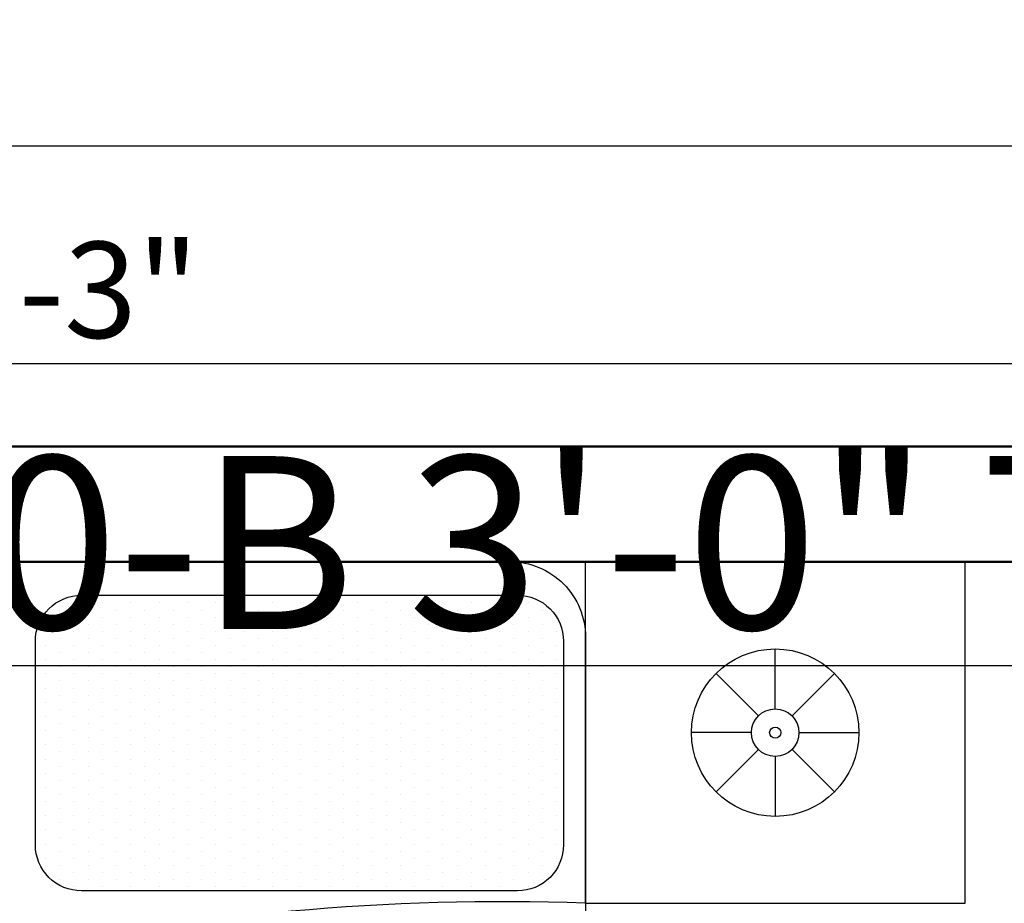
# Model space of a CAD drawing. Units: inches. Extents: x 3064 to 19385, y 846 to 15425.
# Tile 47 of 108: x 5430 to 5481, y 1368 to 1414. Entities that reach past the tile are written whole.
import ezdxf

# ---------------------------------------------------------------- set-up
doc = ezdxf.new("R2010")
doc.units = ezdxf.units.IN
for name, color, linetype, lineweight in [('A-ANNO-DIMS', 2, 'Continuous', 18), ('A-FLOR-FIXT', 9, 'Continuous', 18), ('A-WALL', 7, 'Continuous', 50)]:
    doc.layers.add(name, color=color, linetype=linetype, lineweight=lineweight)
doc.layers.add('BLOCK', color=6, linetype='Continuous')
doc.styles.get("Standard").update_dxf_attribs({"font": 'arial.ttf'})
doc.dimstyles.new('ISO-25', dxfattribs={"dimtxt": 9, "dimasz": 2.5, "dimexe": 1.25, "dimexo": 0.625, "dimtad": 1, "dimdec": 1, "dimlunit": 3, "dimtxsty": 'Standard', "dimcen": 2.5, "dimadec": 0, "dimazin": 0, "dimtfac": 1, "dimtdec": 1, "dimtmove": 0, "dimatfit": 3, "dimfxl": 1, "dimarcsym": 0})

# ---------------------------------------------------------------- blocks, each defined once
blk = doc.blocks.new('*X7')
at = {"color": 0}
for p, q in [((273.9375, 457.03125), (273.9375, 457.03125)), ((274.3125, 457.03125), (274.3125, 457.03125)), ((274.6875, 457.03125), (274.6875, 457.03125)), ((275.0625, 457.03125), (275.0625, 457.03125)), ((275.4375, 457.03125), (275.4375, 457.03125)), ((275.8125, 457.03125), (275.8125, 457.03125)), ((276.1875, 457.03125), (276.1875, 457.03125)), ((276.5625, 457.03125), (276.5625, 457.03125)), ((276.9375, 457.03125), (276.9375, 457.03125)), ((277.3125, 457.03125), (277.3125, 457.03125)), ((277.6875, 457.03125), (277.6875, 457.03125)), ((278.0625, 457.03125), (278.0625, 457.03125)), ((278.4375, 457.03125), (278.4375, 457.03125)), ((278.8125, 457.03125), (278.8125, 457.03125)), ((279.1875, 457.03125), (279.1875, 457.03125)), ((279.5625, 457.03125), (279.5625, 457.03125)), ((273.5625, 456.84375), (273.5625, 456.84375)), ((273.75, 456.9375), (273.75, 456.9375)), ((273.9375, 456.84375), (273.9375, 456.84375)), ((274.125, 456.9375), (274.125, 456.9375)), ((274.3125, 456.84375), (274.3125, 456.84375)), ((274.5, 456.9375), (274.5, 456.9375)), ((274.6875, 456.84375), (274.6875, 456.84375)), ((274.875, 456.9375), (274.875, 456.9375)), ((275.0625, 456.84375), (275.0625, 456.84375)), ((275.25, 456.9375), (275.25, 456.9375)), ((275.4375, 456.84375), (275.4375, 456.84375)), ((275.625, 456.9375), (275.625, 456.9375)), ((275.8125, 456.84375), (275.8125, 456.84375)), ((276, 456.9375), (276, 456.9375)), ((276.1875, 456.84375), (276.1875, 456.84375)), ((276.375, 456.9375), (276.375, 456.9375)), ((276.5625, 456.84375), (276.5625, 456.84375)), ((276.75, 456.9375), (276.75, 456.9375)), ((276.9375, 456.84375), (276.9375, 456.84375)), ((277.125, 456.9375), (277.125, 456.9375)), ((277.3125, 456.84375), (277.3125, 456.84375)), ((277.5, 456.9375), (277.5, 456.9375)), ((277.6875, 456.84375), (277.6875, 456.84375)), ((277.875, 456.9375), (277.875, 456.9375)), ((278.0625, 456.84375), (278.0625, 456.84375)), ((278.25, 456.9375), (278.25, 456.9375)), ((278.4375, 456.84375), (278.4375, 456.84375)), ((278.625, 456.9375), (278.625, 456.9375)), ((278.8125, 456.84375), (278.8125, 456.84375)), ((279, 456.9375), (279, 456.9375)), ((279.1875, 456.84375), (279.1875, 456.84375)), ((279.375, 456.9375), (279.375, 456.9375)), ((279.5625, 456.84375), (279.5625, 456.84375)), ((279.75, 456.9375), (279.75, 456.9375)), ((279.9375, 456.84375), (279.9375, 456.84375)), ((273.375, 456.75), (273.375, 456.75)), ((273.75, 456.75), (273.75, 456.75)), ((274.125, 456.75), (274.125, 456.75)), ((274.5, 456.75), (274.5, 456.75)), ((274.875, 456.75), (274.875, 456.75)), ((275.25, 456.75), (275.25, 456.75)), ((275.625, 456.75), (275.625, 456.75)), ((276, 456.75), (276, 456.75)), ((276.375, 456.75), (276.375, 456.75)), ((276.75, 456.75), (276.75, 456.75)), ((277.125, 456.75), (277.125, 456.75)), ((277.5, 456.75), (277.5, 456.75)), ((277.875, 456.75), (277.875, 456.75)), ((278.25, 456.75), (278.25, 456.75)), ((278.625, 456.75), (278.625, 456.75)), ((279, 456.75), (279, 456.75)), ((279.375, 456.75), (279.375, 456.75)), ((279.75, 456.75), (279.75, 456.75)), ((280.125, 456.75), (280.125, 456.75)), ((273.375, 456.5625), (273.375, 456.5625)), ((273.5625, 456.65625), (273.5625, 456.65625)), ((273.75, 456.5625), (273.75, 456.5625)), ((273.9375, 456.65625), (273.9375, 456.65625)), ((274.125, 456.5625), (274.125, 456.5625)), ((274.3125, 456.65625), (274.3125, 456.65625)), ((274.5, 456.5625), (274.5, 456.5625)), ((274.6875, 456.65625), (274.6875, 456.65625)), ((274.875, 456.5625), (274.875, 456.5625)), ((275.0625, 456.65625), (275.0625, 456.65625)), ((275.25, 456.5625), (275.25, 456.5625)), ((275.4375, 456.65625), (275.4375, 456.65625)), ((275.625, 456.5625), (275.625, 456.5625)), ((275.8125, 456.65625), (275.8125, 456.65625)), ((276, 456.5625), (276, 456.5625)), ((276.1875, 456.65625), (276.1875, 456.65625)), ((276.375, 456.5625), (276.375, 456.5625)), ((276.5625, 456.65625), (276.5625, 456.65625)), ((276.75, 456.5625), (276.75, 456.5625)), ((276.9375, 456.65625), (276.9375, 456.65625)), ((277.125, 456.5625), (277.125, 456.5625)), ((277.3125, 456.65625), (277.3125, 456.65625)), ((277.5, 456.5625), (277.5, 456.5625)), ((277.6875, 456.65625), (277.6875, 456.65625)), ((277.875, 456.5625), (277.875, 456.5625)), ((278.0625, 456.65625), (278.0625, 456.65625)), ((278.25, 456.5625), (278.25, 456.5625)), ((278.4375, 456.65625), (278.4375, 456.65625)), ((278.625, 456.5625), (278.625, 456.5625)), ((278.8125, 456.65625), (278.8125, 456.65625)), ((279, 456.5625), (279, 456.5625)), ((279.1875, 456.65625), (279.1875, 456.65625)), ((279.375, 456.5625), (279.375, 456.5625)), ((279.5625, 456.65625), (279.5625, 456.65625)), ((279.75, 456.5625), (279.75, 456.5625)), ((279.9375, 456.65625), (279.9375, 456.65625)), ((280.125, 456.5625), (280.125, 456.5625)), ((273.5625, 456.46875), (273.5625, 456.46875)), ((273.9375, 456.46875), (273.9375, 456.46875)), ((274.3125, 456.46875), (274.3125, 456.46875)), ((274.6875, 456.46875), (274.6875, 456.46875)), ((275.0625, 456.46875), (275.0625, 456.46875)), ((275.4375, 456.46875), (275.4375, 456.46875)), ((275.8125, 456.46875), (275.8125, 456.46875)), ((276.1875, 456.46875), (276.1875, 456.46875)), ((276.5625, 456.46875), (276.5625, 456.46875)), ((276.9375, 456.46875), (276.9375, 456.46875)), ((277.3125, 456.46875), (277.3125, 456.46875)), ((277.6875, 456.46875), (277.6875, 456.46875)), ((278.0625, 456.46875), (278.0625, 456.46875)), ((278.4375, 456.46875), (278.4375, 456.46875)), ((278.8125, 456.46875), (278.8125, 456.46875)), ((279.1875, 456.46875), (279.1875, 456.46875)), ((279.5625, 456.46875), (279.5625, 456.46875)), ((279.9375, 456.46875), (279.9375, 456.46875)), ((273.375, 456.375), (273.375, 456.375)), ((273.75, 456.375), (273.75, 456.375)), ((274.125, 456.375), (274.125, 456.375)), ((274.5, 456.375), (274.5, 456.375)), ((274.875, 456.375), (274.875, 456.375)), ((275.25, 456.375), (275.25, 456.375)), ((275.625, 456.375), (275.625, 456.375)), ((276, 456.375), (276, 456.375)), ((276.375, 456.375), (276.375, 456.375)), ((276.75, 456.375), (276.75, 456.375)), ((277.125, 456.375), (277.125, 456.375)), ((277.5, 456.375), (277.5, 456.375)), ((277.875, 456.375), (277.875, 456.375)), ((278.25, 456.375), (278.25, 456.375)), ((278.625, 456.375), (278.625, 456.375)), ((279, 456.375), (279, 456.375)), ((279.375, 456.375), (279.375, 456.375)), ((279.75, 456.375), (279.75, 456.375)), ((280.125, 456.375), (280.125, 456.375)), ((273.375, 456.1875), (273.375, 456.1875)), ((273.5625, 456.28125), (273.5625, 456.28125)), ((273.75, 456.1875), (273.75, 456.1875)), ((273.9375, 456.28125), (273.9375, 456.28125)), ((274.125, 456.1875), (274.125, 456.1875)), ((274.3125, 456.28125), (274.3125, 456.28125)), ((274.5, 456.1875), (274.5, 456.1875)), ((274.6875, 456.28125), (274.6875, 456.28125)), ((274.875, 456.1875), (274.875, 456.1875)), ((275.0625, 456.28125), (275.0625, 456.28125)), ((275.25, 456.1875), (275.25, 456.1875)), ((275.4375, 456.28125), (275.4375, 456.28125)), ((275.625, 456.1875), (275.625, 456.1875)), ((275.8125, 456.28125), (275.8125, 456.28125)), ((276, 456.1875), (276, 456.1875)), ((276.1875, 456.28125), (276.1875, 456.28125)), ((276.375, 456.1875), (276.375, 456.1875)), ((276.5625, 456.28125), (276.5625, 456.28125)), ((276.75, 456.1875), (276.75, 456.1875)), ((276.9375, 456.28125), (276.9375, 456.28125)), ((277.125, 456.1875), (277.125, 456.1875)), ((277.3125, 456.28125), (277.3125, 456.28125)), ((277.5, 456.1875), (277.5, 456.1875)), ((277.6875, 456.28125), (277.6875, 456.28125)), ((277.875, 456.1875), (277.875, 456.1875)), ((278.0625, 456.28125), (278.0625, 456.28125)), ((278.25, 456.1875), (278.25, 456.1875)), ((278.4375, 456.28125), (278.4375, 456.28125)), ((278.625, 456.1875), (278.625, 456.1875)), ((278.8125, 456.28125), (278.8125, 456.28125)), ((279, 456.1875), (279, 456.1875)), ((279.1875, 456.28125), (279.1875, 456.28125)), ((279.375, 456.1875), (279.375, 456.1875)), ((279.5625, 456.28125), (279.5625, 456.28125)), ((279.75, 456.1875), (279.75, 456.1875)), ((279.9375, 456.28125), (279.9375, 456.28125)), ((280.125, 456.1875), (280.125, 456.1875)), ((273.5625, 456.09375), (273.5625, 456.09375)), ((273.9375, 456.09375), (273.9375, 456.09375)), ((274.3125, 456.09375), (274.3125, 456.09375)), ((274.6875, 456.09375), (274.6875, 456.09375)), ((275.0625, 456.09375), (275.0625, 456.09375)), ((275.4375, 456.09375), (275.4375, 456.09375)), ((275.8125, 456.09375), (275.8125, 456.09375)), ((276.1875, 456.09375), (276.1875, 456.09375)), ((276.5625, 456.09375), (276.5625, 456.09375)), ((276.9375, 456.09375), (276.9375, 456.09375)), ((277.3125, 456.09375), (277.3125, 456.09375)), ((277.6875, 456.09375), (277.6875, 456.09375)), ((278.0625, 456.09375), (278.0625, 456.09375)), ((278.4375, 456.09375), (278.4375, 456.09375)), ((278.8125, 456.09375), (278.8125, 456.09375)), ((279.1875, 456.09375), (279.1875, 456.09375)), ((279.5625, 456.09375), (279.5625, 456.09375)), ((279.9375, 456.09375), (279.9375, 456.09375)), ((273.375, 456), (273.375, 456)), ((273.75, 456), (273.75, 456)), ((274.125, 456), (274.125, 456)), ((274.5, 456), (274.5, 456)), ((274.875, 456), (274.875, 456)), ((275.25, 456), (275.25, 456)), ((275.625, 456), (275.625, 456)), ((276, 456), (276, 456)), ((276.375, 456), (276.375, 456)), ((276.75, 456), (276.75, 456)), ((277.125, 456), (277.125, 456)), ((277.5, 456), (277.5, 456)), ((277.875, 456), (277.875, 456)), ((278.25, 456), (278.25, 456)), ((278.625, 456), (278.625, 456)), ((279, 456), (279, 456)), ((279.375, 456), (279.375, 456)), ((279.75, 456), (279.75, 456)), ((280.125, 456), (280.125, 456)), ((273.375, 455.8125), (273.375, 455.8125)), ((273.5625, 455.90625), (273.5625, 455.90625)), ((273.75, 455.8125), (273.75, 455.8125)), ((273.9375, 455.90625), (273.9375, 455.90625)), ((274.125, 455.8125), (274.125, 455.8125)), ((274.3125, 455.90625), (274.3125, 455.90625)), ((274.5, 455.8125), (274.5, 455.8125)), ((274.6875, 455.90625), (274.6875, 455.90625)), ((274.875, 455.8125), (274.875, 455.8125)), ((275.0625, 455.90625), (275.0625, 455.90625)), ((275.25, 455.8125), (275.25, 455.8125)), ((275.4375, 455.90625), (275.4375, 455.90625)), ((275.625, 455.8125), (275.625, 455.8125)), ((275.8125, 455.90625), (275.8125, 455.90625)), ((276, 455.8125), (276, 455.8125)), ((276.1875, 455.90625), (276.1875, 455.90625)), ((276.375, 455.8125), (276.375, 455.8125)), ((276.5625, 455.90625), (276.5625, 455.90625)), ((276.75, 455.8125), (276.75, 455.8125)), ((276.9375, 455.90625), (276.9375, 455.90625)), ((277.125, 455.8125), (277.125, 455.8125)), ((277.3125, 455.90625), (277.3125, 455.90625)), ((277.5, 455.8125), (277.5, 455.8125)), ((277.6875, 455.90625), (277.6875, 455.90625)), ((277.875, 455.8125), (277.875, 455.8125)), ((278.0625, 455.90625), (278.0625, 455.90625)), ((278.25, 455.8125), (278.25, 455.8125)), ((278.4375, 455.90625), (278.4375, 455.90625)), ((278.625, 455.8125), (278.625, 455.8125)), ((278.8125, 455.90625), (278.8125, 455.90625)), ((279, 455.8125), (279, 455.8125)), ((279.1875, 455.90625), (279.1875, 455.90625)), ((279.375, 455.8125), (279.375, 455.8125)), ((279.5625, 455.90625), (279.5625, 455.90625)), ((279.75, 455.8125), (279.75, 455.8125)), ((279.9375, 455.90625), (279.9375, 455.90625)), ((280.125, 455.8125), (280.125, 455.8125)), ((273.5625, 455.71875), (273.5625, 455.71875)), ((273.9375, 455.71875), (273.9375, 455.71875)), ((274.3125, 455.71875), (274.3125, 455.71875)), ((274.6875, 455.71875), (274.6875, 455.71875)), ((275.0625, 455.71875), (275.0625, 455.71875)), ((275.4375, 455.71875), (275.4375, 455.71875)), ((275.8125, 455.71875), (275.8125, 455.71875)), ((276.1875, 455.71875), (276.1875, 455.71875)), ((276.5625, 455.71875), (276.5625, 455.71875)), ((276.9375, 455.71875), (276.9375, 455.71875)), ((277.3125, 455.71875), (277.3125, 455.71875)), ((277.6875, 455.71875), (277.6875, 455.71875)), ((278.0625, 455.71875), (278.0625, 455.71875)), ((278.4375, 455.71875), (278.4375, 455.71875)), ((278.8125, 455.71875), (278.8125, 455.71875)), ((279.1875, 455.71875), (279.1875, 455.71875)), ((279.5625, 455.71875), (279.5625, 455.71875)), ((279.9375, 455.71875), (279.9375, 455.71875)), ((273.375, 455.625), (273.375, 455.625)), ((273.5625, 455.53125), (273.5625, 455.53125)), ((273.75, 455.625), (273.75, 455.625)), ((273.9375, 455.53125), (273.9375, 455.53125)), ((274.125, 455.625), (274.125, 455.625)), ((274.3125, 455.53125), (274.3125, 455.53125)), ((274.5, 455.625), (274.5, 455.625)), ((274.6875, 455.53125), (274.6875, 455.53125)), ((274.875, 455.625), (274.875, 455.625)), ((275.0625, 455.53125), (275.0625, 455.53125)), ((275.25, 455.625), (275.25, 455.625)), ((275.4375, 455.53125), (275.4375, 455.53125)), ((275.625, 455.625), (275.625, 455.625)), ((275.8125, 455.53125), (275.8125, 455.53125)), ((276, 455.625), (276, 455.625)), ((276.1875, 455.53125), (276.1875, 455.53125)), ((276.375, 455.625), (276.375, 455.625)), ((276.5625, 455.53125), (276.5625, 455.53125)), ((276.75, 455.625), (276.75, 455.625)), ((276.9375, 455.53125), (276.9375, 455.53125)), ((277.125, 455.625), (277.125, 455.625)), ((277.3125, 455.53125), (277.3125, 455.53125)), ((277.5, 455.625), (277.5, 455.625)), ((277.6875, 455.53125), (277.6875, 455.53125)), ((277.875, 455.625), (277.875, 455.625)), ((278.0625, 455.53125), (278.0625, 455.53125)), ((278.25, 455.625), (278.25, 455.625)), ((278.4375, 455.53125), (278.4375, 455.53125)), ((278.625, 455.625), (278.625, 455.625)), ((278.8125, 455.53125), (278.8125, 455.53125)), ((279, 455.625), (279, 455.625)), ((279.1875, 455.53125), (279.1875, 455.53125)), ((279.375, 455.625), (279.375, 455.625)), ((279.5625, 455.53125), (279.5625, 455.53125)), ((279.75, 455.625), (279.75, 455.625)), ((279.9375, 455.53125), (279.9375, 455.53125)), ((280.125, 455.625), (280.125, 455.625)), ((273.375, 455.4375), (273.375, 455.4375)), ((273.75, 455.4375), (273.75, 455.4375)), ((274.125, 455.4375), (274.125, 455.4375)), ((274.5, 455.4375), (274.5, 455.4375)), ((274.875, 455.4375), (274.875, 455.4375)), ((275.25, 455.4375), (275.25, 455.4375)), ((275.625, 455.4375), (275.625, 455.4375)), ((276, 455.4375), (276, 455.4375)), ((276.375, 455.4375), (276.375, 455.4375)), ((276.75, 455.4375), (276.75, 455.4375)), ((277.125, 455.4375), (277.125, 455.4375)), ((277.5, 455.4375), (277.5, 455.4375)), ((277.875, 455.4375), (277.875, 455.4375)), ((278.25, 455.4375), (278.25, 455.4375)), ((278.625, 455.4375), (278.625, 455.4375)), ((279, 455.4375), (279, 455.4375)), ((279.375, 455.4375), (279.375, 455.4375)), ((279.75, 455.4375), (279.75, 455.4375)), ((280.125, 455.4375), (280.125, 455.4375)), ((273.5625, 455.34375), (273.5625, 455.34375)), ((273.9375, 455.34375), (273.9375, 455.34375)), ((274.3125, 455.34375), (274.3125, 455.34375)), ((274.6875, 455.34375), (274.6875, 455.34375)), ((275.0625, 455.34375), (275.0625, 455.34375)), ((275.4375, 455.34375), (275.4375, 455.34375)), ((275.8125, 455.34375), (275.8125, 455.34375)), ((276.1875, 455.34375), (276.1875, 455.34375)), ((276.5625, 455.34375), (276.5625, 455.34375)), ((276.9375, 455.34375), (276.9375, 455.34375)), ((277.3125, 455.34375), (277.3125, 455.34375)), ((277.6875, 455.34375), (277.6875, 455.34375)), ((278.0625, 455.34375), (278.0625, 455.34375)), ((278.4375, 455.34375), (278.4375, 455.34375)), ((278.8125, 455.34375), (278.8125, 455.34375)), ((279.1875, 455.34375), (279.1875, 455.34375)), ((279.5625, 455.34375), (279.5625, 455.34375)), ((279.9375, 455.34375), (279.9375, 455.34375)), ((273.375, 455.25), (273.375, 455.25)), ((273.5625, 455.15625), (273.5625, 455.15625)), ((273.75, 455.25), (273.75, 455.25)), ((273.9375, 455.15625), (273.9375, 455.15625)), ((274.125, 455.25), (274.125, 455.25)), ((274.3125, 455.15625), (274.3125, 455.15625)), ((274.5, 455.25), (274.5, 455.25)), ((274.6875, 455.15625), (274.6875, 455.15625)), ((274.875, 455.25), (274.875, 455.25)), ((275.0625, 455.15625), (275.0625, 455.15625)), ((275.25, 455.25), (275.25, 455.25)), ((275.4375, 455.15625), (275.4375, 455.15625)), ((275.625, 455.25), (275.625, 455.25)), ((275.8125, 455.15625), (275.8125, 455.15625)), ((276, 455.25), (276, 455.25)), ((276.1875, 455.15625), (276.1875, 455.15625)), ((276.375, 455.25), (276.375, 455.25)), ((276.5625, 455.15625), (276.5625, 455.15625)), ((276.75, 455.25), (276.75, 455.25)), ((276.9375, 455.15625), (276.9375, 455.15625)), ((277.125, 455.25), (277.125, 455.25)), ((277.3125, 455.15625), (277.3125, 455.15625)), ((277.5, 455.25), (277.5, 455.25)), ((277.6875, 455.15625), (277.6875, 455.15625)), ((277.875, 455.25), (277.875, 455.25)), ((278.0625, 455.15625), (278.0625, 455.15625)), ((278.25, 455.25), (278.25, 455.25)), ((278.4375, 455.15625), (278.4375, 455.15625)), ((278.625, 455.25), (278.625, 455.25)), ((278.8125, 455.15625), (278.8125, 455.15625)), ((279, 455.25), (279, 455.25)), ((279.1875, 455.15625), (279.1875, 455.15625)), ((279.375, 455.25), (279.375, 455.25)), ((279.5625, 455.15625), (279.5625, 455.15625)), ((279.75, 455.25), (279.75, 455.25)), ((279.9375, 455.15625), (279.9375, 455.15625)), ((280.125, 455.25), (280.125, 455.25)), ((273.375, 455.0625), (273.375, 455.0625)), ((273.75, 455.0625), (273.75, 455.0625)), ((274.125, 455.0625), (274.125, 455.0625)), ((274.5, 455.0625), (274.5, 455.0625)), ((274.875, 455.0625), (274.875, 455.0625)), ((275.25, 455.0625), (275.25, 455.0625)), ((275.625, 455.0625), (275.625, 455.0625)), ((276, 455.0625), (276, 455.0625)), ((276.375, 455.0625), (276.375, 455.0625)), ((276.75, 455.0625), (276.75, 455.0625)), ((277.125, 455.0625), (277.125, 455.0625)), ((277.5, 455.0625), (277.5, 455.0625)), ((277.875, 455.0625), (277.875, 455.0625)), ((278.25, 455.0625), (278.25, 455.0625)), ((278.625, 455.0625), (278.625, 455.0625)), ((279, 455.0625), (279, 455.0625)), ((279.375, 455.0625), (279.375, 455.0625)), ((279.75, 455.0625), (279.75, 455.0625)), ((280.125, 455.0625), (280.125, 455.0625)), ((273.375, 454.875), (273.375, 454.875)), ((273.5625, 454.96875), (273.5625, 454.96875)), ((273.75, 454.875), (273.75, 454.875)), ((273.9375, 454.96875), (273.9375, 454.96875)), ((274.125, 454.875), (274.125, 454.875)), ((274.3125, 454.96875), (274.3125, 454.96875)), ((274.5, 454.875), (274.5, 454.875)), ((274.6875, 454.96875), (274.6875, 454.96875)), ((274.875, 454.875), (274.875, 454.875)), ((275.0625, 454.96875), (275.0625, 454.96875)), ((275.25, 454.875), (275.25, 454.875)), ((275.4375, 454.96875), (275.4375, 454.96875)), ((275.625, 454.875), (275.625, 454.875)), ((275.8125, 454.96875), (275.8125, 454.96875)), ((276, 454.875), (276, 454.875)), ((276.1875, 454.96875), (276.1875, 454.96875)), ((276.375, 454.875), (276.375, 454.875)), ((276.5625, 454.96875), (276.5625, 454.96875)), ((276.75, 454.875), (276.75, 454.875)), ((276.9375, 454.96875), (276.9375, 454.96875)), ((277.125, 454.875), (277.125, 454.875)), ((277.3125, 454.96875), (277.3125, 454.96875)), ((277.5, 454.875), (277.5, 454.875)), ((277.6875, 454.96875), (277.6875, 454.96875)), ((277.875, 454.875), (277.875, 454.875)), ((278.0625, 454.96875), (278.0625, 454.96875)), ((278.25, 454.875), (278.25, 454.875)), ((278.4375, 454.96875), (278.4375, 454.96875)), ((278.625, 454.875), (278.625, 454.875)), ((278.8125, 454.96875), (278.8125, 454.96875)), ((279, 454.875), (279, 454.875)), ((279.1875, 454.96875), (279.1875, 454.96875)), ((279.375, 454.875), (279.375, 454.875)), ((279.5625, 454.96875), (279.5625, 454.96875)), ((279.75, 454.875), (279.75, 454.875)), ((279.9375, 454.96875), (279.9375, 454.96875)), ((280.125, 454.875), (280.125, 454.875)), ((273.5625, 454.78125), (273.5625, 454.78125)), ((273.9375, 454.78125), (273.9375, 454.78125)), ((274.3125, 454.78125), (274.3125, 454.78125)), ((274.6875, 454.78125), (274.6875, 454.78125)), ((275.0625, 454.78125), (275.0625, 454.78125)), ((275.4375, 454.78125), (275.4375, 454.78125)), ((275.8125, 454.78125), (275.8125, 454.78125)), ((276.1875, 454.78125), (276.1875, 454.78125)), ((276.5625, 454.78125), (276.5625, 454.78125)), ((276.9375, 454.78125), (276.9375, 454.78125)), ((277.3125, 454.78125), (277.3125, 454.78125)), ((277.6875, 454.78125), (277.6875, 454.78125)), ((278.0625, 454.78125), (278.0625, 454.78125)), ((278.4375, 454.78125), (278.4375, 454.78125)), ((278.8125, 454.78125), (278.8125, 454.78125)), ((279.1875, 454.78125), (279.1875, 454.78125)), ((279.5625, 454.78125), (279.5625, 454.78125)), ((279.9375, 454.78125), (279.9375, 454.78125)), ((273.375, 454.6875), (273.375, 454.6875)), ((273.75, 454.6875), (273.75, 454.6875)), ((274.125, 454.6875), (274.125, 454.6875)), ((274.5, 454.6875), (274.5, 454.6875)), ((274.875, 454.6875), (274.875, 454.6875)), ((275.25, 454.6875), (275.25, 454.6875)), ((275.625, 454.6875), (275.625, 454.6875)), ((276, 454.6875), (276, 454.6875)), ((276.375, 454.6875), (276.375, 454.6875)), ((276.75, 454.6875), (276.75, 454.6875)), ((277.125, 454.6875), (277.125, 454.6875)), ((277.5, 454.6875), (277.5, 454.6875)), ((277.875, 454.6875), (277.875, 454.6875)), ((278.25, 454.6875), (278.25, 454.6875)), ((278.625, 454.6875), (278.625, 454.6875)), ((279, 454.6875), (279, 454.6875)), ((279.375, 454.6875), (279.375, 454.6875)), ((279.75, 454.6875), (279.75, 454.6875)), ((280.125, 454.6875), (280.125, 454.6875)), ((273.375, 454.5), (273.375, 454.5)), ((273.5625, 454.59375), (273.5625, 454.59375)), ((273.75, 454.5), (273.75, 454.5)), ((273.9375, 454.59375), (273.9375, 454.59375)), ((274.125, 454.5), (274.125, 454.5)), ((274.3125, 454.59375), (274.3125, 454.59375)), ((274.5, 454.5), (274.5, 454.5)), ((274.6875, 454.59375), (274.6875, 454.59375)), ((274.875, 454.5), (274.875, 454.5)), ((275.0625, 454.59375), (275.0625, 454.59375)), ((275.25, 454.5), (275.25, 454.5)), ((275.4375, 454.59375), (275.4375, 454.59375)), ((275.625, 454.5), (275.625, 454.5)), ((275.8125, 454.59375), (275.8125, 454.59375)), ((276, 454.5), (276, 454.5)), ((276.1875, 454.59375), (276.1875, 454.59375)), ((276.375, 454.5), (276.375, 454.5)), ((276.5625, 454.59375), (276.5625, 454.59375)), ((276.75, 454.5), (276.75, 454.5)), ((276.9375, 454.59375), (276.9375, 454.59375)), ((277.125, 454.5), (277.125, 454.5)), ((277.3125, 454.59375), (277.3125, 454.59375)), ((277.5, 454.5), (277.5, 454.5)), ((277.6875, 454.59375), (277.6875, 454.59375)), ((277.875, 454.5), (277.875, 454.5)), ((278.0625, 454.59375), (278.0625, 454.59375)), ((278.25, 454.5), (278.25, 454.5)), ((278.4375, 454.59375), (278.4375, 454.59375)), ((278.625, 454.5), (278.625, 454.5)), ((278.8125, 454.59375), (278.8125, 454.59375)), ((279, 454.5), (279, 454.5)), ((279.1875, 454.59375), (279.1875, 454.59375)), ((279.375, 454.5), (279.375, 454.5)), ((279.5625, 454.59375), (279.5625, 454.59375)), ((279.75, 454.5), (279.75, 454.5)), ((279.9375, 454.59375), (279.9375, 454.59375)), ((280.125, 454.5), (280.125, 454.5)), ((273.5625, 454.40625), (273.5625, 454.40625)), ((273.9375, 454.40625), (273.9375, 454.40625)), ((274.3125, 454.40625), (274.3125, 454.40625)), ((274.6875, 454.40625), (274.6875, 454.40625)), ((275.0625, 454.40625), (275.0625, 454.40625)), ((275.4375, 454.40625), (275.4375, 454.40625)), ((275.8125, 454.40625), (275.8125, 454.40625)), ((276.1875, 454.40625), (276.1875, 454.40625)), ((276.5625, 454.40625), (276.5625, 454.40625)), ((276.9375, 454.40625), (276.9375, 454.40625)), ((277.3125, 454.40625), (277.3125, 454.40625)), ((277.6875, 454.40625), (277.6875, 454.40625)), ((278.0625, 454.40625), (278.0625, 454.40625)), ((278.4375, 454.40625), (278.4375, 454.40625)), ((278.8125, 454.40625), (278.8125, 454.40625)), ((279.1875, 454.40625), (279.1875, 454.40625)), ((279.5625, 454.40625), (279.5625, 454.40625)), ((279.9375, 454.40625), (279.9375, 454.40625)), ((273.375, 454.3125), (273.375, 454.3125)), ((273.75, 454.3125), (273.75, 454.3125)), ((274.125, 454.3125), (274.125, 454.3125)), ((274.5, 454.3125), (274.5, 454.3125)), ((274.875, 454.3125), (274.875, 454.3125)), ((275.25, 454.3125), (275.25, 454.3125)), ((275.625, 454.3125), (275.625, 454.3125)), ((276, 454.3125), (276, 454.3125)), ((276.375, 454.3125), (276.375, 454.3125)), ((276.75, 454.3125), (276.75, 454.3125)), ((277.125, 454.3125), (277.125, 454.3125)), ((277.5, 454.3125), (277.5, 454.3125)), ((277.875, 454.3125), (277.875, 454.3125)), ((278.25, 454.3125), (278.25, 454.3125)), ((278.625, 454.3125), (278.625, 454.3125)), ((279, 454.3125), (279, 454.3125)), ((279.375, 454.3125), (279.375, 454.3125)), ((279.75, 454.3125), (279.75, 454.3125)), ((280.125, 454.3125), (280.125, 454.3125)), ((273.375, 454.125), (273.375, 454.125)), ((273.5625, 454.21875), (273.5625, 454.21875)), ((273.75, 454.125), (273.75, 454.125)), ((273.9375, 454.21875), (273.9375, 454.21875)), ((274.125, 454.125), (274.125, 454.125)), ((274.3125, 454.21875), (274.3125, 454.21875)), ((274.5, 454.125), (274.5, 454.125)), ((274.6875, 454.21875), (274.6875, 454.21875)), ((274.875, 454.125), (274.875, 454.125)), ((275.0625, 454.21875), (275.0625, 454.21875)), ((275.25, 454.125), (275.25, 454.125)), ((275.4375, 454.21875), (275.4375, 454.21875)), ((275.625, 454.125), (275.625, 454.125)), ((275.8125, 454.21875), (275.8125, 454.21875)), ((276, 454.125), (276, 454.125)), ((276.1875, 454.21875), (276.1875, 454.21875)), ((276.375, 454.125), (276.375, 454.125)), ((276.5625, 454.21875), (276.5625, 454.21875)), ((276.75, 454.125), (276.75, 454.125)), ((276.9375, 454.21875), (276.9375, 454.21875)), ((277.125, 454.125), (277.125, 454.125)), ((277.3125, 454.21875), (277.3125, 454.21875)), ((277.5, 454.125), (277.5, 454.125)), ((277.6875, 454.21875), (277.6875, 454.21875)), ((277.875, 454.125), (277.875, 454.125)), ((278.0625, 454.21875), (278.0625, 454.21875)), ((278.25, 454.125), (278.25, 454.125)), ((278.4375, 454.21875), (278.4375, 454.21875)), ((278.625, 454.125), (278.625, 454.125)), ((278.8125, 454.21875), (278.8125, 454.21875)), ((279, 454.125), (279, 454.125)), ((279.1875, 454.21875), (279.1875, 454.21875)), ((279.375, 454.125), (279.375, 454.125)), ((279.5625, 454.21875), (279.5625, 454.21875)), ((279.75, 454.125), (279.75, 454.125)), ((279.9375, 454.21875), (279.9375, 454.21875)), ((280.125, 454.125), (280.125, 454.125)), ((273.5625, 454.03125), (273.5625, 454.03125)), ((273.9375, 454.03125), (273.9375, 454.03125)), ((274.3125, 454.03125), (274.3125, 454.03125)), ((274.6875, 454.03125), (274.6875, 454.03125)), ((275.0625, 454.03125), (275.0625, 454.03125)), ((275.4375, 454.03125), (275.4375, 454.03125)), ((275.8125, 454.03125), (275.8125, 454.03125)), ((276.1875, 454.03125), (276.1875, 454.03125)), ((276.5625, 454.03125), (276.5625, 454.03125)), ((276.9375, 454.03125), (276.9375, 454.03125)), ((277.3125, 454.03125), (277.3125, 454.03125)), ((277.6875, 454.03125), (277.6875, 454.03125)), ((278.0625, 454.03125), (278.0625, 454.03125)), ((278.4375, 454.03125), (278.4375, 454.03125)), ((278.8125, 454.03125), (278.8125, 454.03125)), ((279.1875, 454.03125), (279.1875, 454.03125)), ((279.5625, 454.03125), (279.5625, 454.03125)), ((279.9375, 454.03125), (279.9375, 454.03125)), ((273.375, 453.9375), (273.375, 453.9375)), ((273.5625, 453.84375), (273.5625, 453.84375)), ((273.75, 453.9375), (273.75, 453.9375)), ((273.9375, 453.84375), (273.9375, 453.84375)), ((274.125, 453.9375), (274.125, 453.9375)), ((274.3125, 453.84375), (274.3125, 453.84375)), ((274.5, 453.9375), (274.5, 453.9375)), ((274.6875, 453.84375), (274.6875, 453.84375)), ((274.875, 453.9375), (274.875, 453.9375)), ((275.0625, 453.84375), (275.0625, 453.84375)), ((275.25, 453.9375), (275.25, 453.9375)), ((275.4375, 453.84375), (275.4375, 453.84375)), ((275.625, 453.9375), (275.625, 453.9375)), ((275.8125, 453.84375), (275.8125, 453.84375)), ((276, 453.9375), (276, 453.9375)), ((276.1875, 453.84375), (276.1875, 453.84375)), ((276.375, 453.9375), (276.375, 453.9375)), ((276.5625, 453.84375), (276.5625, 453.84375)), ((276.75, 453.9375), (276.75, 453.9375)), ((276.9375, 453.84375), (276.9375, 453.84375)), ((277.125, 453.9375), (277.125, 453.9375)), ((277.3125, 453.84375), (277.3125, 453.84375)), ((277.5, 453.9375), (277.5, 453.9375)), ((277.6875, 453.84375), (277.6875, 453.84375)), ((277.875, 453.9375), (277.875, 453.9375)), ((278.0625, 453.84375), (278.0625, 453.84375)), ((278.25, 453.9375), (278.25, 453.9375)), ((278.4375, 453.84375), (278.4375, 453.84375)), ((278.625, 453.9375), (278.625, 453.9375)), ((278.8125, 453.84375), (278.8125, 453.84375)), ((279, 453.9375), (279, 453.9375)), ((279.1875, 453.84375), (279.1875, 453.84375)), ((279.375, 453.9375), (279.375, 453.9375)), ((279.5625, 453.84375), (279.5625, 453.84375)), ((279.75, 453.9375), (279.75, 453.9375)), ((279.9375, 453.84375), (279.9375, 453.84375)), ((280.125, 453.9375), (280.125, 453.9375)), ((273.375, 453.75), (273.375, 453.75)), ((273.75, 453.75), (273.75, 453.75)), ((274.125, 453.75), (274.125, 453.75)), ((274.5, 453.75), (274.5, 453.75)), ((274.875, 453.75), (274.875, 453.75)), ((275.25, 453.75), (275.25, 453.75)), ((275.625, 453.75), (275.625, 453.75)), ((276, 453.75), (276, 453.75)), ((276.375, 453.75), (276.375, 453.75)), ((276.75, 453.75), (276.75, 453.75)), ((277.125, 453.75), (277.125, 453.75)), ((277.5, 453.75), (277.5, 453.75)), ((277.875, 453.75), (277.875, 453.75)), ((278.25, 453.75), (278.25, 453.75)), ((278.625, 453.75), (278.625, 453.75)), ((279, 453.75), (279, 453.75)), ((279.375, 453.75), (279.375, 453.75)), ((279.75, 453.75), (279.75, 453.75)), ((280.125, 453.75), (280.125, 453.75)), ((273.5625, 453.65625), (273.5625, 453.65625)), ((273.9375, 453.65625), (273.9375, 453.65625)), ((274.3125, 453.65625), (274.3125, 453.65625)), ((274.6875, 453.65625), (274.6875, 453.65625)), ((275.0625, 453.65625), (275.0625, 453.65625)), ((275.4375, 453.65625), (275.4375, 453.65625)), ((275.8125, 453.65625), (275.8125, 453.65625)), ((276.1875, 453.65625), (276.1875, 453.65625)), ((276.5625, 453.65625), (276.5625, 453.65625)), ((276.9375, 453.65625), (276.9375, 453.65625)), ((277.3125, 453.65625), (277.3125, 453.65625)), ((277.6875, 453.65625), (277.6875, 453.65625)), ((278.0625, 453.65625), (278.0625, 453.65625)), ((278.4375, 453.65625), (278.4375, 453.65625)), ((278.8125, 453.65625), (278.8125, 453.65625)), ((279.1875, 453.65625), (279.1875, 453.65625)), ((279.5625, 453.65625), (279.5625, 453.65625)), ((279.9375, 453.65625), (279.9375, 453.65625)), ((273.375, 453.5625), (273.375, 453.5625)), ((273.5625, 453.46875), (273.5625, 453.46875)), ((273.75, 453.5625), (273.75, 453.5625)), ((273.9375, 453.46875), (273.9375, 453.46875)), ((274.125, 453.5625), (274.125, 453.5625)), ((274.3125, 453.46875), (274.3125, 453.46875)), ((274.5, 453.5625), (274.5, 453.5625)), ((274.6875, 453.46875), (274.6875, 453.46875)), ((274.875, 453.5625), (274.875, 453.5625)), ((275.0625, 453.46875), (275.0625, 453.46875)), ((275.25, 453.5625), (275.25, 453.5625)), ((275.4375, 453.46875), (275.4375, 453.46875)), ((275.625, 453.5625), (275.625, 453.5625)), ((275.8125, 453.46875), (275.8125, 453.46875)), ((276, 453.5625), (276, 453.5625)), ((276.1875, 453.46875), (276.1875, 453.46875)), ((276.375, 453.5625), (276.375, 453.5625)), ((276.5625, 453.46875), (276.5625, 453.46875)), ((276.75, 453.5625), (276.75, 453.5625)), ((276.9375, 453.46875), (276.9375, 453.46875)), ((277.125, 453.5625), (277.125, 453.5625)), ((277.3125, 453.46875), (277.3125, 453.46875)), ((277.5, 453.5625), (277.5, 453.5625)), ((277.6875, 453.46875), (277.6875, 453.46875)), ((277.875, 453.5625), (277.875, 453.5625)), ((278.0625, 453.46875), (278.0625, 453.46875)), ((278.25, 453.5625), (278.25, 453.5625)), ((278.4375, 453.46875), (278.4375, 453.46875)), ((278.625, 453.5625), (278.625, 453.5625)), ((278.8125, 453.46875), (278.8125, 453.46875)), ((279, 453.5625), (279, 453.5625)), ((279.1875, 453.46875), (279.1875, 453.46875)), ((279.375, 453.5625), (279.375, 453.5625)), ((279.5625, 453.46875), (279.5625, 453.46875)), ((279.75, 453.5625), (279.75, 453.5625)), ((279.9375, 453.46875), (279.9375, 453.46875)), ((280.125, 453.5625), (280.125, 453.5625)), ((273.375, 453.375), (273.375, 453.375)), ((273.75, 453.375), (273.75, 453.375)), ((274.125, 453.375), (274.125, 453.375)), ((274.5, 453.375), (274.5, 453.375)), ((274.875, 453.375), (274.875, 453.375)), ((275.25, 453.375), (275.25, 453.375)), ((275.625, 453.375), (275.625, 453.375)), ((276, 453.375), (276, 453.375)), ((276.375, 453.375), (276.375, 453.375)), ((276.75, 453.375), (276.75, 453.375)), ((277.125, 453.375), (277.125, 453.375)), ((277.5, 453.375), (277.5, 453.375)), ((277.875, 453.375), (277.875, 453.375)), ((278.25, 453.375), (278.25, 453.375)), ((278.625, 453.375), (278.625, 453.375)), ((279, 453.375), (279, 453.375)), ((279.375, 453.375), (279.375, 453.375)), ((279.75, 453.375), (279.75, 453.375)), ((273.5625, 453.28125), (273.5625, 453.28125)), ((273.75, 453.1875), (273.75, 453.1875)), ((273.9375, 453.28125), (273.9375, 453.28125)), ((274.125, 453.1875), (274.125, 453.1875)), ((274.3125, 453.28125), (274.3125, 453.28125)), ((274.5, 453.1875), (274.5, 453.1875)), ((274.6875, 453.28125), (274.6875, 453.28125)), ((274.875, 453.1875), (274.875, 453.1875)), ((275.0625, 453.28125), (275.0625, 453.28125)), ((275.25, 453.1875), (275.25, 453.1875)), ((275.4375, 453.28125), (275.4375, 453.28125)), ((275.625, 453.1875), (275.625, 453.1875)), ((275.8125, 453.28125), (275.8125, 453.28125)), ((276, 453.1875), (276, 453.1875)), ((276.1875, 453.28125), (276.1875, 453.28125)), ((276.375, 453.1875), (276.375, 453.1875)), ((276.5625, 453.28125), (276.5625, 453.28125)), ((276.75, 453.1875), (276.75, 453.1875)), ((276.9375, 453.28125), (276.9375, 453.28125)), ((277.125, 453.1875), (277.125, 453.1875)), ((277.3125, 453.28125), (277.3125, 453.28125)), ((277.5, 453.1875), (277.5, 453.1875)), ((277.6875, 453.28125), (277.6875, 453.28125)), ((277.875, 453.1875), (277.875, 453.1875)), ((278.0625, 453.28125), (278.0625, 453.28125)), ((278.25, 453.1875), (278.25, 453.1875)), ((278.4375, 453.28125), (278.4375, 453.28125)), ((278.625, 453.1875), (278.625, 453.1875)), ((278.8125, 453.28125), (278.8125, 453.28125)), ((279, 453.1875), (279, 453.1875)), ((279.1875, 453.28125), (279.1875, 453.28125)), ((279.375, 453.1875), (279.375, 453.1875)), ((279.5625, 453.28125), (279.5625, 453.28125)), ((279.75, 453.1875), (279.75, 453.1875)), ((279.9375, 453.28125), (279.9375, 453.28125))]:
    blk.add_line(p, q, dxfattribs=at)
blk = doc.blocks.new('A$C52E67D0D')
at = {"layer": 'BLOCK'}
for p, q in [((2251.5, 1605.5), (2251.5, 1684.7)), ((2229.3, 1596.3), (2173.3, 1652.3)), ((2273.7, 1596.3), (2329.7, 1652.3)), ((2220.1, 1574.1), (2140.9, 1574.1)), ((2282.9, 1574.1), (2362.1, 1574.1)), ((2229.3, 1551.9), (2173.3, 1495.9)), ((2273.7, 1551.9), (2329.7, 1495.9)), ((2251.5, 1542.8), (2251.5, 1463.5))]:
    blk.add_line(p, q, dxfattribs=at)
for points in [[(1901, 0), (601, 0, -0.414214), (501, 100), (501, 1700, -0.414214), (601, 1800), (1901, 1800, -0.414214), (2001, 1700), (2001, 100, -0.414214)], [(1911, 1365.1), (1335, 1365.1, -0.414214), (1274.2, 1425.9), (1274.2, 1694.8, -0.414214), (1335, 1755.7), (1911, 1755.7, -0.414214), (1971.8, 1694.8), (1971.8, 1425.9, -0.414214)]]:
    blk.add_lwpolyline(points, format="xyb", close=True, dxfattribs=at)
blk.add_lwpolyline([(2001, 1348.6), (2001, 1799.6), (2502, 1799.6), (2502, 1348.6)], close=True, dxfattribs=at)
for radius in [110.6, 31.4, 7.46]:
    blk.add_circle((2251.5, 1574.1), radius, dxfattribs=at)
blk.add_arc((1888.6, -1664.5), 3015.3, 87.8642, 117.4001, dxfattribs=at)
at = {"layer": 'BLOCK', "xscale": 100, "yscale": 100, "zscale": 100}
blk.add_blockref('*X7', (-26050, -43948.2), dxfattribs=at)
blk = doc.blocks.new('*D92')
at = {"layer": 'A-ANNO-DIMS', "color": 0, "lineweight": -2, "transparency": 16777216}
for p, q in [((5332.017, 1392.721), (5332.017, 1397.658)), ((5527.017, 1392.721), (5527.017, 1397.658)), ((5334.517, 1396.408), (5524.517, 1396.408))]:
    blk.add_line(p, q, dxfattribs=at)
at = {"layer": 'A-ANNO-DIMS', "color": 0, "transparency": 16777216}
for points in [[(5334.517, 1396.825), (5334.517, 1395.992), (5332.017, 1396.408)], [(5524.517, 1396.825), (5524.517, 1395.992), (5527.017, 1396.408)]]:
    blk.add_solid(points, dxfattribs=at)
at = {"layer": 'Defpoints', "color": 0, "transparency": 16777216}
for p in [(5527.017, 1396.408), (5332.017, 1392.096), (5527.017, 1392.096)]:
    blk.add_point(p, dxfattribs=at)
at = {"layer": 'A-ANNO-DIMS', "color": 0, "transparency": 16777216, "insert": (5429.517, 1399.588), "char_height": 5, "attachment_point": 5}
blk.add_mtext('16\'-3"', dxfattribs=at)
blk = doc.blocks.new('*D94')
at = {"layer": 'A-ANNO-DIMS', "color": 0, "lineweight": -2, "transparency": 16777216}
for p, q in [((5191.017, 1392.721), (5191.017, 1408.956)), ((5533.017, 1392.721), (5533.017, 1408.956)), ((5530.517, 1407.706), (5193.517, 1407.706))]:
    blk.add_line(p, q, dxfattribs=at)
at = {"layer": 'A-ANNO-DIMS', "color": 0, "transparency": 16777216}
for points in [[(5193.517, 1408.122), (5193.517, 1407.289), (5191.017, 1407.706)], [(5530.517, 1408.122), (5530.517, 1407.289), (5533.017, 1407.706)]]:
    blk.add_solid(points, dxfattribs=at)
at = {"layer": 'Defpoints', "color": 0, "transparency": 16777216}
for p in [(5191.017, 1407.706), (5191.017, 1392.096), (5533.017, 1392.096)]:
    blk.add_point(p, dxfattribs=at)
at = {"layer": 'A-ANNO-DIMS', "color": 0, "transparency": 16777216, "insert": (5362.017, 1410.884), "char_height": 5, "attachment_point": 5}
blk.add_mtext('28\'-6"', dxfattribs=at)
blk = doc.blocks.new('*D443')
at = {"layer": 'A-ANNO-DIMS', "color": 0, "lineweight": -2, "transparency": 16777216}
for p, q in [((5356.017, 1385.471), (5356.017, 1379.446)), ((5392.017, 1385.471), (5392.017, 1379.446)), ((5358.517, 1380.696), (5389.517, 1380.696)), ((5392.017, 1380.696), (5506.898, 1380.696))]:
    blk.add_line(p, q, dxfattribs=at)
at = {"layer": 'A-ANNO-DIMS', "color": 0, "transparency": 16777216}
for points in [[(5358.517, 1381.113), (5358.517, 1380.28), (5356.017, 1380.696)], [(5389.517, 1381.113), (5389.517, 1380.28), (5392.017, 1380.696)]]:
    blk.add_solid(points, dxfattribs=at)
at = {"layer": 'Defpoints', "color": 0, "transparency": 16777216}
for p in [(5356.017, 1386.096), (5392.017, 1386.096), (5392.017, 1380.696)]:
    blk.add_point(p, dxfattribs=at)
at = {"layer": 'A-ANNO-DIMS', "color": 0, "transparency": 16777216, "insert": (5450.707, 1385.92), "char_height": 9, "attachment_point": 5}
blk.add_mtext('W1000-B 3\'-0" TYP.', dxfattribs=at)

msp = doc.modelspace()

# ---------------------------------------------------------------- linework, layer by layer
at = {"layer": 'A-WALL'}
for p, q in [((5533.017, 1392.096), (5191.017, 1392.096)), ((5527.017, 1386.096), (5332.017, 1386.096))]:
    msp.add_line(p, q, dxfattribs=at)

# ---------------------------------------------------------------- block references
at = {"layer": 'A-FLOR-FIXT', "xscale": 0.039370099999992, "yscale": 0.039370099999992, "zscale": 0.039370099999992}
msp.add_blockref('A$C52E67D0D', (5380.265, 1315.23), dxfattribs=at)

# ---------------------------------------------------------------- dimensions: what is measured, and where the dimension line sits
at = {"layer": 'A-ANNO-DIMS'}
for base, p1, p2, override, picture, middle in [((5191.017, 1407.706), (5533.017, 1392.096), (5191.017, 1392.096), {"dimtxt": 5, "dimclrd": 0, "dimclre": 0, "dimclrt": 0}, '*D94', (5362.017, 1410.884)), ((5527.017, 1396.408), (5332.017, 1392.096), (5527.017, 1392.096), {"dimtxt": 5, "dimclrd": 0, "dimclre": 0, "dimclrt": 0, "dimtmove": 1}, '*D92', (5429.517, 1399.588))]:
    dim = msp.add_linear_dim(base=base, p1=p1, p2=p2, dimstyle='ISO-25', override=override, dxfattribs=at)
    dim.commit()
    dim.dimension.update_dxf_attribs({"geometry": picture, "text_midpoint": middle})
dim = msp.add_linear_dim(base=(5392.017, 1380.696), p1=(5356.017, 1386.096), p2=(5392.017, 1386.096), text='W1000-B <> TYP.', dimstyle='ISO-25', override={"dimdec": 1, "dimrnd": 0, "dimzin": 1, "dimlunit": 4, "dimfrac": 2}, dxfattribs=at)
dim.commit()
dim.dimension.update_dxf_attribs({"geometry": '*D443', "text_midpoint": (5450.707, 1385.92)})

doc.saveas('drawing.dxf')
